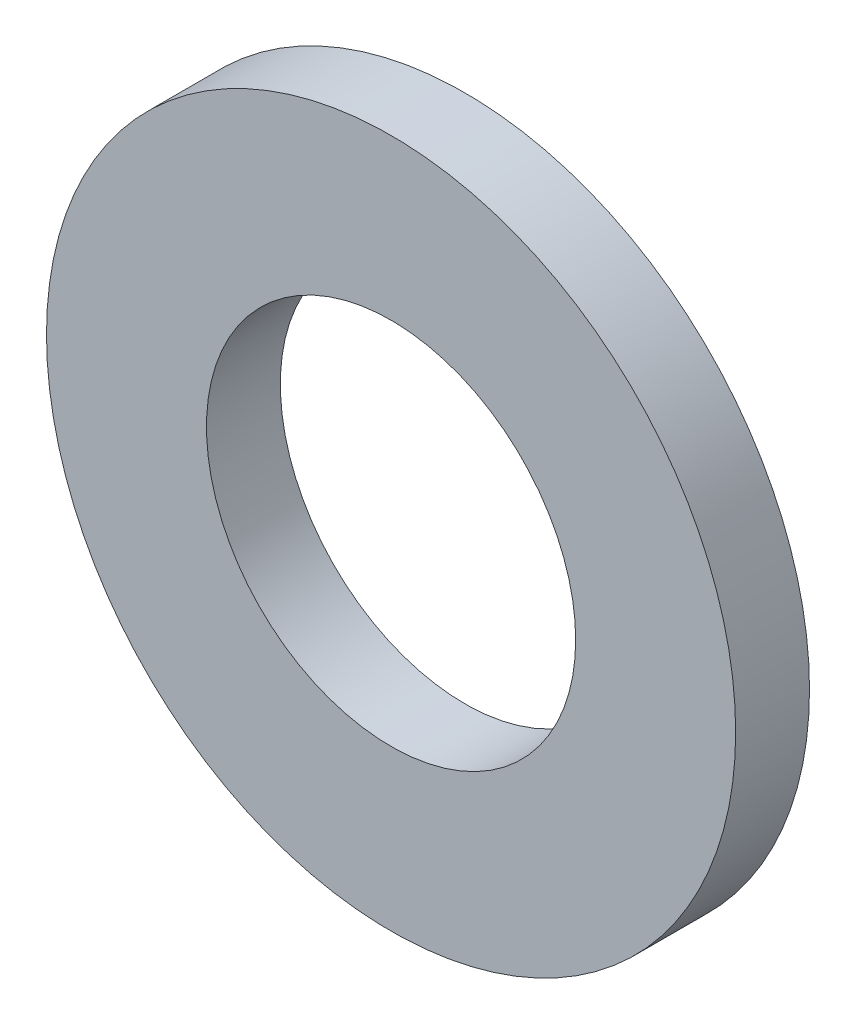
ISO-10303-21;
HEADER;
FILE_DESCRIPTION(('STEP AP214'),'2;1');
FILE_NAME('part.step','',(''),(''),'','','');
FILE_SCHEMA(('AUTOMOTIVE_DESIGN { 1 0 10303 214 1 1 1 1 }'));
ENDSEC;
DATA;
#1=APPLICATION_CONTEXT('core data for automotive mechanical design processes');
#2=APPLICATION_PROTOCOL_DEFINITION('international standard','automotive_design',2000,#1);
#3=PRODUCT_CONTEXT('',#1,'mechanical');
#4=PRODUCT('Part','Part','',(#3));
#5=PRODUCT_RELATED_PRODUCT_CATEGORY('part','',(#4));
#6=PRODUCT_DEFINITION_FORMATION('','',#4);
#7=PRODUCT_DEFINITION_CONTEXT('part definition',#1,'design');
#8=PRODUCT_DEFINITION('design','',#6,#7);
#9=PRODUCT_DEFINITION_SHAPE('','',#8);
#10=(LENGTH_UNIT() NAMED_UNIT(*) SI_UNIT(.MILLI.,.METRE.));
#11=(NAMED_UNIT(*) PLANE_ANGLE_UNIT() SI_UNIT($,.RADIAN.));
#12=(NAMED_UNIT(*) SI_UNIT($,.STERADIAN.) SOLID_ANGLE_UNIT());
#13=UNCERTAINTY_MEASURE_WITH_UNIT(LENGTH_MEASURE(1.E-05),#10,'distance_accuracy_value','');
#14=(GEOMETRIC_REPRESENTATION_CONTEXT(3) GLOBAL_UNCERTAINTY_ASSIGNED_CONTEXT((#13)) GLOBAL_UNIT_ASSIGNED_CONTEXT((#10,
#11,#12)) REPRESENTATION_CONTEXT('',''));
#15=CARTESIAN_POINT('',(0.,0.,0.));
#16=DIRECTION('',(0.,0.,1.));
#17=DIRECTION('',(1.,0.,0.));
#18=AXIS2_PLACEMENT_3D('',#15,#16,#17);
#19=CARTESIAN_POINT('',(0.,0.,1.5));
#20=DIRECTION('',(0.,0.,1.));
#21=DIRECTION('',(1.,0.,0.));
#22=AXIS2_PLACEMENT_3D('',#19,#20,#21);
#23=PLANE('',#22);
#24=CARTESIAN_POINT('',(0.,0.,1.5));
#25=DIRECTION('',(0.,0.,1.));
#26=DIRECTION('',(1.,0.,0.));
#27=AXIS2_PLACEMENT_3D('',#24,#25,#26);
#28=CIRCLE('',#27,14.);
#29=CARTESIAN_POINT('',(14.,0.,1.5));
#30=VERTEX_POINT('',#29);
#31=EDGE_CURVE('E10',#30,#30,#28,.T.);
#32=ORIENTED_EDGE('',*,*,#31,.T.);
#33=EDGE_LOOP('',(#32));
#34=FACE_BOUND('',#33,.T.);
#35=CARTESIAN_POINT('',(0.,0.,1.5));
#36=DIRECTION('',(0.,0.,1.));
#37=DIRECTION('',(1.,0.,0.));
#38=AXIS2_PLACEMENT_3D('',#35,#36,#37);
#39=CIRCLE('',#38,7.5);
#40=CARTESIAN_POINT('',(7.5,0.,1.5));
#41=VERTEX_POINT('',#40);
#42=EDGE_CURVE('E53',#41,#41,#39,.T.);
#43=ORIENTED_EDGE('',*,*,#42,.F.);
#44=EDGE_LOOP('',(#43));
#45=FACE_BOUND('',#44,.T.);
#46=ADVANCED_FACE('F43',(#34,#45),#23,.T.);
#47=CARTESIAN_POINT('',(0.,0.,-1.5));
#48=DIRECTION('',(0.,0.,1.));
#49=DIRECTION('',(1.,0.,0.));
#50=AXIS2_PLACEMENT_3D('',#47,#48,#49);
#51=PLANE('',#50);
#52=CARTESIAN_POINT('',(0.,0.,-1.5));
#53=DIRECTION('',(0.,0.,1.));
#54=DIRECTION('',(1.,0.,0.));
#55=AXIS2_PLACEMENT_3D('',#52,#53,#54);
#56=CIRCLE('',#55,14.);
#57=CARTESIAN_POINT('',(14.,0.,-1.5));
#58=VERTEX_POINT('',#57);
#59=EDGE_CURVE('E50',#58,#58,#56,.T.);
#60=ORIENTED_EDGE('',*,*,#59,.F.);
#61=EDGE_LOOP('',(#60));
#62=FACE_BOUND('',#61,.T.);
#63=CARTESIAN_POINT('',(0.,0.,-1.5));
#64=DIRECTION('',(0.,0.,1.));
#65=DIRECTION('',(1.,0.,0.));
#66=AXIS2_PLACEMENT_3D('',#63,#64,#65);
#67=CIRCLE('',#66,7.5);
#68=CARTESIAN_POINT('',(7.5,0.,-1.5));
#69=VERTEX_POINT('',#68);
#70=EDGE_CURVE('E57',#69,#69,#67,.T.);
#71=ORIENTED_EDGE('',*,*,#70,.T.);
#72=EDGE_LOOP('',(#71));
#73=FACE_BOUND('',#72,.T.);
#74=ADVANCED_FACE('F67',(#62,#73),#51,.F.);
#75=CARTESIAN_POINT('',(0.,0.,1.5));
#76=DIRECTION('',(0.,0.,-1.));
#77=DIRECTION('',(-1.,0.,0.));
#78=AXIS2_PLACEMENT_3D('',#75,#76,#77);
#79=CYLINDRICAL_SURFACE('',#78,14.);
#80=ORIENTED_EDGE('',*,*,#31,.F.);
#81=EDGE_LOOP('',(#80));
#82=FACE_BOUND('',#81,.T.);
#83=ORIENTED_EDGE('',*,*,#59,.T.);
#84=EDGE_LOOP('',(#83));
#85=FACE_BOUND('',#84,.T.);
#86=ADVANCED_FACE('F44',(#82,#85),#79,.T.);
#87=CARTESIAN_POINT('',(0.,0.,1.5));
#88=DIRECTION('',(0.,0.,-1.));
#89=DIRECTION('',(-1.,0.,0.));
#90=AXIS2_PLACEMENT_3D('',#87,#88,#89);
#91=CYLINDRICAL_SURFACE('',#90,7.5);
#92=ORIENTED_EDGE('',*,*,#42,.T.);
#93=EDGE_LOOP('',(#92));
#94=FACE_BOUND('',#93,.T.);
#95=ORIENTED_EDGE('',*,*,#70,.F.);
#96=EDGE_LOOP('',(#95));
#97=FACE_BOUND('',#96,.T.);
#98=ADVANCED_FACE('F64',(#94,#97),#91,.F.);
#99=CLOSED_SHELL('',(#46,#74,#86,#98));
#100=MANIFOLD_SOLID_BREP('B2',#99);
#101=ADVANCED_BREP_SHAPE_REPRESENTATION('',(#18,#100),#14);
#102=SHAPE_DEFINITION_REPRESENTATION(#9,#101);
ENDSEC;
END-ISO-10303-21;
